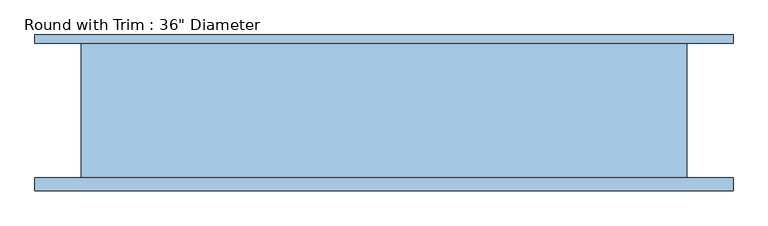
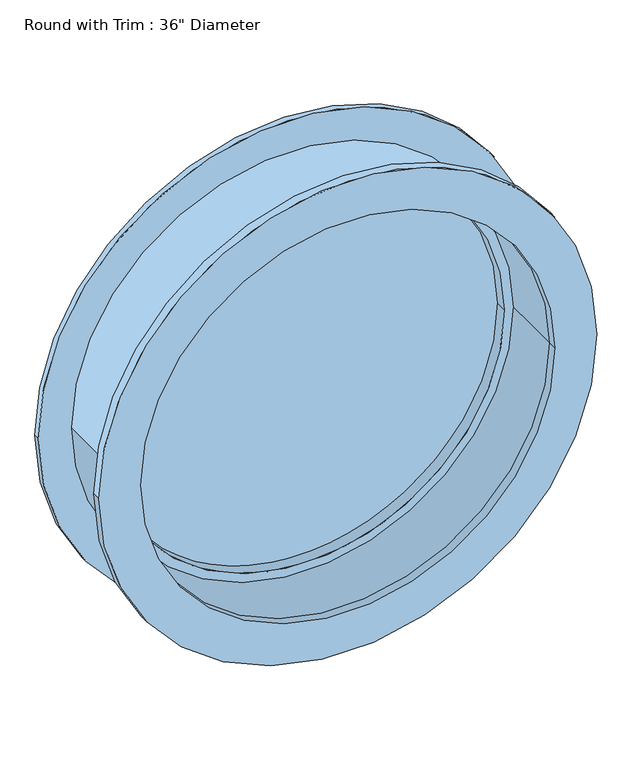
"""IFC4 building model written with IfcOpenShell, lengths in millimetres: window geometry."""

from ifc_helpers import new_model, si_unit, point, frame, frame_2d, origin, place, context, project, spatial, circle_curve, trimmed, segment, composite_curve, outline, extrude, source, transform, mapped, element, save


def window_736d8d37(model_context):
    return source(origin(), model_context, "Body", "SweptSolid", [
        extrude(outline(composite_curve([segment(trimmed(circle_curve(frame_2d((1219.2, 0.0)), 527.05), [point((1219.2, -527.05))], [point((1219.2, 527.05))], False, "CARTESIAN"), True, "CONTINUOUS"), segment(trimmed(circle_curve(frame_2d((1219.2, 0.0)), 527.05), [point((1219.2, 527.05))], [point((1219.2, -527.05))], False, "CARTESIAN"), True, "CONTINUOUS")], self_intersect=False), holes=[composite_curve([segment(trimmed(circle_curve(frame_2d((1219.2, 0.0)), 438.15), [point((1219.2, -438.15))], [point((1219.2, 438.15))], True, "CARTESIAN"), True, "CONTINUOUS"), segment(trimmed(circle_curve(frame_2d((1219.2, 0.0)), 438.15), [point((1219.2, 438.15))], [point((1219.2, -438.15))], True, "CARTESIAN"), True, "CONTINUOUS")], self_intersect=False)]), frame((0.0, -120.65, 0.0), z_axis=(0.0, 1.0, 0.0), x_axis=(0.0, 0.0, 1.0)), (0.0, 0.0, 1.0), 19.05),
        extrude(outline(composite_curve([segment(trimmed(circle_curve(frame_2d((1219.2, 0.0)), 527.05), [point((1219.2, -527.05))], [point((1219.2, 527.05))], False, "CARTESIAN"), True, "CONTINUOUS"), segment(trimmed(circle_curve(frame_2d((1219.2, 0.0)), 527.05), [point((1219.2, 527.05))], [point((1219.2, -527.05))], False, "CARTESIAN"), True, "CONTINUOUS")], self_intersect=False), holes=[composite_curve([segment(trimmed(circle_curve(frame_2d((1219.2, 0.0)), 438.15), [point((1219.2, -438.15))], [point((1219.2, 438.15))], True, "CARTESIAN"), True, "CONTINUOUS"), segment(trimmed(circle_curve(frame_2d((1219.2, 0.0)), 438.15), [point((1219.2, 438.15))], [point((1219.2, -438.15))], True, "CARTESIAN"), True, "CONTINUOUS")], self_intersect=False)]), frame((0.0, 101.6, 0.0), z_axis=(0.0, 1.0, 0.0), x_axis=(0.0, 0.0, 1.0)), (0.0, 0.0, 1.0), 12.7),
        extrude(outline(composite_curve([segment(trimmed(circle_curve(frame_2d((1219.2, 0.0)), 419.1), [point((1219.2, -419.1))], [point((1219.2, 419.1))], False, "CARTESIAN"), True, "CONTINUOUS"), segment(trimmed(circle_curve(frame_2d((1219.2, 0.0)), 419.1), [point((1219.2, 419.1))], [point((1219.2, -419.1))], False, "CARTESIAN"), True, "CONTINUOUS")], self_intersect=False)), frame((0.0, 57.15, 0.0), z_axis=(0.0, 1.0, 0.0), x_axis=(0.0, 0.0, 1.0)), (0.0, 0.0, 1.0), 12.7),
        extrude(outline(composite_curve([segment(trimmed(circle_curve(frame_2d((1219.2, 0.0)), 438.15), [point((1219.2, -438.15))], [point((1219.2, 438.15))], False, "CARTESIAN"), True, "CONTINUOUS"), segment(trimmed(circle_curve(frame_2d((1219.2, 0.0)), 438.15), [point((1219.2, 438.15))], [point((1219.2, -438.15))], False, "CARTESIAN"), True, "CONTINUOUS")], self_intersect=False), holes=[composite_curve([segment(trimmed(circle_curve(frame_2d((1219.2, 0.0)), 419.1), [point((1219.2, -419.1))], [point((1219.2, 419.1))], True, "CARTESIAN"), True, "CONTINUOUS"), segment(trimmed(circle_curve(frame_2d((1219.2, 0.0)), 419.1), [point((1219.2, 419.1))], [point((1219.2, -419.1))], True, "CARTESIAN"), True, "CONTINUOUS")], self_intersect=False)]), frame((0.0, 31.75, 0.0), z_axis=(0.0, 1.0, 0.0), x_axis=(0.0, 0.0, 1.0)), (0.0, 0.0, 1.0), 50.8),
        extrude(outline(composite_curve([segment(trimmed(circle_curve(frame_2d((1219.2, 0.0)), 457.2), [point((1219.2, -457.2))], [point((1219.2, 457.2))], False, "CARTESIAN"), True, "CONTINUOUS"), segment(trimmed(circle_curve(frame_2d((1219.2, 0.0)), 457.2), [point((1219.2, 457.2))], [point((1219.2, -457.2))], False, "CARTESIAN"), True, "CONTINUOUS")], self_intersect=False), holes=[composite_curve([segment(trimmed(circle_curve(frame_2d((1219.2, 0.0)), 438.15), [point((1219.2, -438.15))], [point((1219.2, 438.15))], True, "CARTESIAN"), True, "CONTINUOUS"), segment(trimmed(circle_curve(frame_2d((1219.2, 0.0)), 438.15), [point((1219.2, 438.15))], [point((1219.2, -438.15))], True, "CARTESIAN"), True, "CONTINUOUS")], self_intersect=False)]), frame((0.0, -101.6, 0.0), z_axis=(0.0, 1.0, 0.0), x_axis=(0.0, 0.0, 1.0)), (0.0, 0.0, 1.0), 203.2),
    ])


if __name__ == "__main__":
    model = new_model("IFC4")
    model_context = context("Model", 3, world=origin())
    ifc_project = project(units=[si_unit("LENGTHUNIT", "METRE", prefix="MILLI")], contexts=[model_context])
    site = spatial("IfcSite", under=ifc_project)
    building = spatial("IfcBuilding", under=site)
    placement = place(None, origin())
    window_shape = window_736d8d37(model_context)
    element("IfcWindow", 1, ObjectType="Round with Trim : 36\" Diameter", at=placement, inside=building, context=model_context, shape_type="MappedRepresentation", body=[
        mapped(window_shape, transform((0.0, 0.0, 0.0), x_axis=(1.0, 0.0, 0.0), y_axis=(0.0, 1.0, 0.0), z_axis=(0.0, 0.0, 1.0))),
    ])
    save(model, "model.ifc")

# Revit data of these elements
# Type "Round with Trim : 36\" Diameter"
#   Type Mark = "27"
#   Construction Type Id = "GSP4R"
#   Assembly Code = "B2020100"
#   Analytic Construction = "1/8 in Pilkington single glazing"
#   Visual Light Transmittance = 0.9
#   Solar Heat Gain Coefficient = 0.78
#   Heat Transfer Coefficient (U) = 0.6496 BTU/(h·ft²·°F)
#   Default Sill Height = 2' - 6"
#   Trim Projection - Ext. = 0' - 0 1/2"
#   Trim Projection - Int. = 0' - 0 3/4"
#   Trim Width - Exterior = 0' - 3 1/2"
#   Trim Width - Interior = 0' - 3 1/2"
#   Width = 3' - 0"
#   Define Thermal Properties by = 1
#   Glass Pane Material = Glass
#   Sash Material = Sash
#   Trim Exterior Material = Trim
#   Trim Interior Material = Trim
#   Wall Closure = (empty or 0)
# Element 1 (IfcWindow, "Round with Trim : 36\" Diameter")
#   Materials on its faces: "Trim", "Sash", "Glass"
# Materials
#   "Glass": class "Glass", colour RGB 0 128 192, transparency 0.75, Description = "Soda Lime Glass", Cost = 0
#   "Sash": class "Wood", colour RGB 224 178 126, transparency 0
#   "Trim": class "Wood", colour RGB 224 178 126, transparency 0
